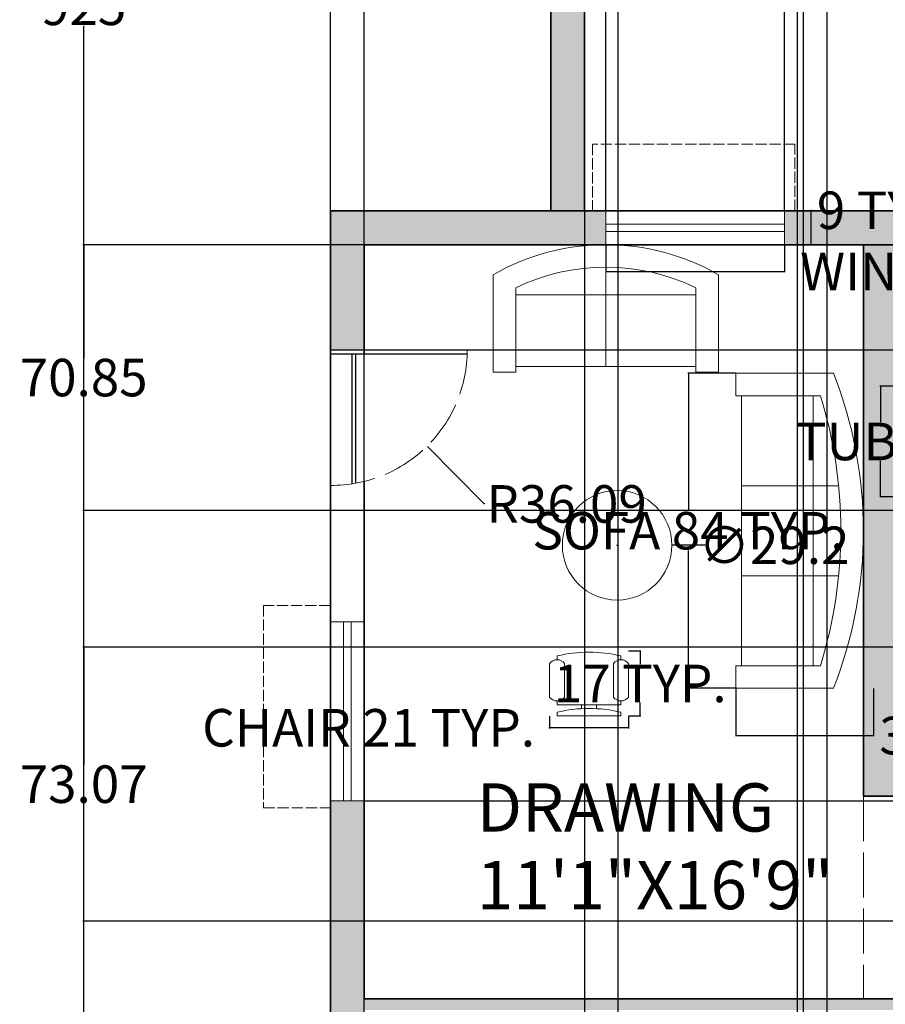
# Model space of a CAD drawing. Units: inches. Extents: x 300 to 1007, y 2 to 1069.
# Tile 4 of 12: x 337 to 568, y 271 to 533. Entities that reach past the tile are written whole.
import ezdxf

# ---------------------------------------------------------------- set-up
doc = ezdxf.new("R2010")
doc.units = ezdxf.units.IN
doc.header["$MEASUREMENT"] = 0
doc.linetypes.add('ACAD_ISO02W100', pattern=[15, 12, -3])
for name, color, linetype, lineweight in [('A-ANNO-DIMS', 2, 'Continuous', 18), ('A-AREA-IDEN', 7, 'Continuous', 18), ('A-DOOR', 3, 'Continuous', 25), ('A-DOOR-SWNG', 3, 'ACAD_ISO02W100', 13), ('A-FLOR-SLAB', 7, 'Continuous', 35), ('A-FURN', 8, 'Continuous', 18), ('A-GLAZ', 4, 'Continuous', 18), ('A-GLAZ-OVHD', 8, 'ACAD_ISO02W100', 13), ('A-WALL', 7, 'Continuous', 35), ('A-WALL-OVHD', 8, 'ACAD_ISO02W100', 18)]:
    doc.layers.add(name, color=color, linetype=linetype, lineweight=lineweight)
doc.layers.add('A-WALL-PATT', color=9, linetype='Continuous', lineweight=9, true_color=0xc7c8ca)
doc.styles.get("Standard").update_dxf_attribs({"font": 'arial.ttf'})
doc.dimstyles.get("Standard").update_dxf_attribs({"dimtxt": 10, "dimasz": 0.18, "dimexe": 0.18, "dimexo": 0.0625, "dimgap": 0.09, "dimtad": 0, "dimtih": 1, "dimtoh": 1, "dimdec": 0, "dimzin": 0, "dimdsep": 46, "dimlunit": 3, "dimtxsty": 'Standard', "dimcen": 0.09, "dimadec": 0, "dimazin": 0, "dimtfac": 1, "dimtdec": 0, "dimtofl": 0, "dimtmove": 0, "dimatfit": 3, "dimfxl": 1, "dimtolj": 1, "dimtzin": 0, "dimarcsym": 0})

# ---------------------------------------------------------------- blocks, each defined once
blk = doc.blocks.new('Chair - Desk')
for p, q in [((-8.5, 0), (-8.5, -1)), ((-8.5, 0), (8.5, 0)), ((8.5, 0), (8.5, -1)), ((-2, -3), (-2, -1.9355)), ((2, -1.9576), (2, -3)), ((-10.5, -5), (-10.5, -14)), ((-8.5, -3), (-8.5, -4)), ((-8.5, -3), (8.5, -3)), ((-6.5, -14), (-6.5, -5)), ((6.5, -5), (6.5, -14)), ((8.5, -3), (8.5, -4)), ((10.5, -14), (10.5, -5)), ((-8.5, -15), (-8.5, -16)), ((8.5, -15), (8.5, -16))]:
    blk.add_line(p, q)
for centre, radius, start, end in [((0, 34.625), 36.625, 256.5803, 283.4197), ((-8.5, -6.5), 2.5, 36.8699, 143.1301), ((8.5, -6.5), 2.5, 36.8699, 143.1301), ((-8.5, -12.5), 2.5, 216.8699, 323.1301), ((8.5, -12.5), 2.5, 216.8699, 323.1301), ((0, 19.625), 36.625, 256.5803, 283.4197)]:
    blk.add_arc(centre, radius, start, end)
blk = doc.blocks.new('Sofa - Roundback Loveseat 5 ft.')
for p, q in [((0, -32.44198), (0, -5.99998)), ((-24, -33.99998), (-24, -11.46958)), ((24.00004, -33.99998), (24.00004, -11.46958)), ((-23.9998, -13.38178), (23.99986, -13.38178)), ((-24, -32.44198), (24.00004, -32.44198))]:
    blk.add_line(p, q)
for points in [[(-24, -33.99998), (-30, -33.99998), (-30, -7.99998)], [(30.00004, -7.99998), (30.00004, -33.99998), (24.00004, -33.99998)]]:
    blk.add_lwpolyline(points)
for centre, radius, start, end in [((0, -60.24998), 60.24998, 60.13715, 119.8628), ((0, -61.38438), 55.38444, 64.32083, 115.6792)]:
    blk.add_arc(centre, radius, start, end)
blk = doc.blocks.new('Sofa - Roundback 7 ft.')
for p, q in [((-12.00002, -32.4421), (-12.00003, -6.5971)), ((11.99997, -32.4421), (11.99998, -6.5971)), ((-36.000027, -34), (-36.000027, -11.4696)), ((35.99998, -34), (35.99998, -11.4696)), ((-35.999844, -13.3819), (35.9998, -13.3819)), ((-36.000027, -32.4421), (35.99998, -32.4421))]:
    blk.add_line(p, q)
for points in [[(-36.000027, -34), (-42.000027, -34), (-42.000027, -8)], [(41.99998, -8), (41.99998, -34), (35.99998, -34)]]:
    blk.add_lwpolyline(points)
for centre, radius, start, end in [((0, -114.25), 114.25, 68.43141, 111.5686), ((-0.00001, -127.1968), 121.1968, 72.72033, 107.2797)]:
    blk.add_arc(centre, radius, start, end)
blk = doc.blocks.new('WIN-48')
for p, q in [((-47.83, 0), (-47.83, 4.5)), ((-47.83, 4.5), (-47.83, -4.5)), ((0, 4.5), (0, -4.5)), ((0, 1), (-47.83, 1)), ((0, -1), (-47.83, -1))]:
    blk.add_line(p, q)
blk = doc.blocks.new('WIN-47_5-8')
for p, q in [((-47.61, 0), (-47.61, 4.5)), ((-47.61, 4.5), (-47.61, -4.5)), ((0, -4.5), (0, 4.5)), ((0, 1), (-47.61, 1)), ((0, -1), (-47.61, -1))]:
    blk.add_line(p, q)
blk = doc.blocks.new('WINDOW-HOOD-54')
at = {"ltscale": 0.25}
for p, q in [((0, 17.83), (-53.97, 17.83)), ((-53.97, 17.83), (-53.97, 0)), ((0, 0), (0, 17.83))]:
    blk.add_line(p, q, dxfattribs=at)
blk = doc.blocks.new('*D21')
at = {"layer": 'A-ANNO-DIMS', "color": 0, "lineweight": -2, "transparency": 16777216}
for p, q in [((478.51, 347.69), (478.51, 344.42)), ((499.51, 347.69), (499.51, 344.42)), ((478.51, 344.6), (478.33, 344.6)), ((499.33, 344.6), (478.69, 344.6))]:
    blk.add_line(p, q, dxfattribs=at)
at = {"layer": 'A-ANNO-DIMS', "color": 0, "transparency": 16777216}
for points in [[(478.69, 344.63), (478.69, 344.57), (478.51, 344.6)], [(499.33, 344.63), (499.33, 344.57), (499.51, 344.6)]]:
    blk.add_solid(points, dxfattribs=at)
at = {"layer": 'Defpoints', "color": 0, "transparency": 16777216}
for p in [(478.51, 347.75), (499.51, 347.75), (478.51, 344.6)]:
    blk.add_point(p, dxfattribs=at)
at = {"layer": 'A-ANNO-DIMS', "color": 0, "transparency": 16777216, "insert": (430.29, 344.6), "char_height": 10, "attachment_point": 5}
blk.add_mtext('\\A1;CHAIR 21 TYP.', dxfattribs=at)
blk = doc.blocks.new('*D22')
at = {"layer": 'A-ANNO-DIMS', "color": 0, "lineweight": -2, "transparency": 16777216}
for p, q in [((499.57, 365.08), (502.84, 365.08)), ((502.66, 364.9), (502.66, 361.53)), ((502.66, 347.93), (502.66, 351.3)), ((499.57, 347.75), (502.84, 347.75))]:
    blk.add_line(p, q, dxfattribs=at)
at = {"layer": 'A-ANNO-DIMS', "color": 0, "transparency": 16777216}
for points in [[(502.63, 364.9), (502.69, 364.9), (502.66, 365.08)], [(502.63, 347.93), (502.69, 347.93), (502.66, 347.75)]]:
    blk.add_solid(points, dxfattribs=at)
at = {"layer": 'Defpoints', "color": 0, "transparency": 16777216}
for p in [(499.51, 365.08), (499.51, 347.75), (502.66, 347.75)]:
    blk.add_point(p, dxfattribs=at)
at = {"layer": 'A-ANNO-DIMS', "color": 0, "transparency": 16777216, "insert": (502.66, 356.42), "char_height": 10, "attachment_point": 5}
blk.add_mtext('\\A1;17 TYP.', dxfattribs=at)
blk = doc.blocks.new('*D35')
at = {"layer": 'A-ANNO-DIMS', "color": 0, "lineweight": -2, "transparency": 16777216}
for p, q in [((571.06, 435.66), (566.52, 435.66)), ((566.7, 435.48), (566.7, 426.11)), ((566.7, 406.35), (566.7, 415.72)), ((571.06, 406.17), (566.52, 406.17))]:
    blk.add_line(p, q, dxfattribs=at)
at = {"layer": 'A-ANNO-DIMS', "color": 0, "transparency": 16777216}
for points in [[(566.67, 435.48), (566.73, 435.48), (566.7, 435.66)], [(566.67, 406.35), (566.73, 406.35), (566.7, 406.17)]]:
    blk.add_solid(points, dxfattribs=at)
at = {"layer": 'Defpoints', "color": 0, "transparency": 16777216}
for p in [(571.12, 435.66), (566.7, 406.17), (571.12, 406.17)]:
    blk.add_point(p, dxfattribs=at)
at = {"layer": 'A-ANNO-DIMS', "color": 0, "transparency": 16777216, "insert": (566.7, 420.92), "char_height": 10, "attachment_point": 5}
blk.add_mtext('\\A1;TUB 29', dxfattribs=at)
blk = doc.blocks.new('*D51')
at = {"layer": 'A-ANNO-DIMS', "color": 0, "lineweight": -2, "transparency": 16777216}
for p, q in [((528.06, 439.13), (515.34, 439.13)), ((515.52, 438.95), (515.52, 402.39)), ((515.52, 355.31), (515.52, 391.86)), ((528.06, 355.13), (515.34, 355.13))]:
    blk.add_line(p, q, dxfattribs=at)
at = {"layer": 'A-ANNO-DIMS', "color": 0, "transparency": 16777216}
for points in [[(515.49, 438.95), (515.55, 438.95), (515.52, 439.13)], [(515.49, 355.31), (515.55, 355.31), (515.52, 355.13)]]:
    blk.add_solid(points, dxfattribs=at)
at = {"layer": 'Defpoints', "color": 0, "transparency": 16777216}
for p in [(528.12, 439.13), (515.52, 355.13), (528.12, 355.13)]:
    blk.add_point(p, dxfattribs=at)
at = {"layer": 'A-ANNO-DIMS', "color": 0, "transparency": 16777216, "insert": (515.52, 397.13), "char_height": 10, "attachment_point": 5}
blk.add_mtext('\\A1;SOFA 84 TYP.', dxfattribs=at)
blk = doc.blocks.new('*D52')
at = {"layer": 'A-ANNO-DIMS', "color": 0, "lineweight": -2, "transparency": 16777216}
for p, q in [((528.12, 355.06), (528.12, 342.35)), ((564.79, 355.06), (564.79, 342.35)), ((528.3, 342.53), (564.61, 342.53)), ((564.79, 342.53), (564.97, 342.53))]:
    blk.add_line(p, q, dxfattribs=at)
at = {"layer": 'A-ANNO-DIMS', "color": 0, "transparency": 16777216}
for points in [[(528.3, 342.56), (528.3, 342.5), (528.12, 342.53)], [(564.61, 342.56), (564.61, 342.5), (564.79, 342.53)]]:
    blk.add_solid(points, dxfattribs=at)
at = {"layer": 'Defpoints', "color": 0, "transparency": 16777216}
for p in [(528.12, 355.13), (564.79, 355.13), (564.79, 342.53)]:
    blk.add_point(p, dxfattribs=at)
at = {"layer": 'A-ANNO-DIMS', "color": 0, "transparency": 16777216, "insert": (589.39, 342.53), "char_height": 10, "attachment_point": 5}
blk.add_mtext('\\A1;37 TYP.', dxfattribs=at)
blk = doc.blocks.new('*D55')
at = {"layer": 'A-ANNO-DIMS', "color": 0, "lineweight": -2, "transparency": 16777216}
for p, q in [((493.48, 473.32), (493.48, 466.06)), ((541.08, 473.32), (541.08, 466.06)), ((493.66, 466.24), (540.9, 466.24)), ((541.08, 466.24), (541.26, 466.24))]:
    blk.add_line(p, q, dxfattribs=at)
at = {"layer": 'A-ANNO-DIMS', "color": 0, "transparency": 16777216}
for points in [[(493.66, 466.27), (493.66, 466.21), (493.48, 466.24)], [(540.9, 466.27), (540.9, 466.21), (541.08, 466.24)]]:
    blk.add_solid(points, dxfattribs=at)
at = {"layer": 'Defpoints', "color": 0, "transparency": 16777216}
for p in [(493.48, 473.38), (541.08, 473.38), (541.08, 466.24)]:
    blk.add_point(p, dxfattribs=at)
at = {"layer": 'A-ANNO-DIMS', "color": 0, "transparency": 16777216, "insert": (598.48, 466.24), "char_height": 10, "attachment_point": 5}
blk.add_mtext('\\A1;WINDOW 48 TYP.', dxfattribs=at)
blk = doc.blocks.new('*D56')
at = {"layer": 'A-ANNO-DIMS', "color": 0, "lineweight": -2, "transparency": 16777216}
for p, q in [((541.14, 482.38), (548.4, 482.38)), ((548.22, 482.38), (548.22, 482.56)), ((548.22, 482.56), (548.4, 482.56)), ((548.22, 473.56), (548.22, 482.2)), ((541.14, 473.38), (548.4, 473.38))]:
    blk.add_line(p, q, dxfattribs=at)
at = {"layer": 'A-ANNO-DIMS', "color": 0, "transparency": 16777216}
for points in [[(548.19, 482.2), (548.25, 482.2), (548.22, 482.38)], [(548.19, 473.56), (548.25, 473.56), (548.22, 473.38)]]:
    blk.add_solid(points, dxfattribs=at)
at = {"layer": 'Defpoints', "color": 0, "transparency": 16777216}
for p in [(541.08, 482.38), (548.22, 482.38), (541.08, 473.38)]:
    blk.add_point(p, dxfattribs=at)
at = {"layer": 'A-ANNO-DIMS', "color": 0, "transparency": 16777216, "insert": (568.95, 482.56), "char_height": 10, "attachment_point": 5}
blk.add_mtext('\\A1;9 TYP.', dxfattribs=at)
blk = doc.blocks.new('*D74')
at = {"layer": 'A-ANNO-DIMS', "color": 0, "lineweight": -2, "transparency": 16777216}
for p, q in [((478.76, 999.45), (354.19, 999.45)), ((354.37, 999.27), (354.37, 542.11)), ((354.37, 74.56), (354.37, 531.72)), ((420.06, 74.38), (354.19, 74.38))]:
    blk.add_line(p, q, dxfattribs=at)
at = {"layer": 'A-ANNO-DIMS', "color": 0, "transparency": 16777216}
for points in [[(354.34, 999.27), (354.4, 999.27), (354.37, 999.45)], [(354.34, 74.56), (354.4, 74.56), (354.37, 74.38)]]:
    blk.add_solid(points, dxfattribs=at)
at = {"layer": 'Defpoints', "color": 0, "transparency": 16777216}
for p in [(354.37, 999.45), (478.83, 999.45), (420.12, 74.38)]:
    blk.add_point(p, dxfattribs=at)
at = {"layer": 'A-ANNO-DIMS', "color": 0, "transparency": 16777216, "insert": (354.37, 536.92), "char_height": 10, "attachment_point": 5}
blk.add_mtext('\\A1;925', dxfattribs=at)
blk = doc.blocks.new('*D79')
at = {"layer": 'A-ANNO-DIMS', "color": 0, "lineweight": -2, "transparency": 16777216}
for p, q in [((420.12, 482.45), (420.12, 1063.03)), ((420.3, 1062.85), (436.4, 1062.85)), ((478.65, 1062.85), (462.55, 1062.85)), ((478.83, 482.45), (478.83, 1063.03))]:
    blk.add_line(p, q, dxfattribs=at)
at = {"layer": 'A-ANNO-DIMS', "color": 0, "transparency": 16777216}
for points in [[(420.3, 1062.88), (420.3, 1062.82), (420.12, 1062.85)], [(478.65, 1062.88), (478.65, 1062.82), (478.83, 1062.85)]]:
    blk.add_solid(points, dxfattribs=at)
at = {"layer": 'Defpoints', "color": 0, "transparency": 16777216}
for p in [(478.83, 1062.85), (420.12, 482.38), (478.83, 482.38)]:
    blk.add_point(p, dxfattribs=at)
at = {"layer": 'A-ANNO-DIMS', "color": 0, "transparency": 16777216, "insert": (449.47, 1062.85), "char_height": 10, "attachment_point": 5}
blk.add_mtext('\\A1;58.7', dxfattribs=at)
blk = doc.blocks.new('*D88')
at = {"layer": 'A-ANNO-DIMS', "color": 0, "lineweight": -2, "transparency": 16777216}
for p, q in [((429.12, 83.45), (429.12, 1063.03)), ((429.3, 1062.85), (445.92, 1062.85)), ((496.59, 1062.85), (479.97, 1062.85)), ((496.77, 83.45), (496.77, 1063.03))]:
    blk.add_line(p, q, dxfattribs=at)
at = {"layer": 'A-ANNO-DIMS', "color": 0, "transparency": 16777216}
for points in [[(429.3, 1062.88), (429.3, 1062.82), (429.12, 1062.85)], [(496.59, 1062.88), (496.59, 1062.82), (496.77, 1062.85)]]:
    blk.add_solid(points, dxfattribs=at)
at = {"layer": 'Defpoints', "color": 0, "transparency": 16777216}
for p in [(496.77, 1062.85), (429.12, 83.38), (496.77, 83.38)]:
    blk.add_point(p, dxfattribs=at)
at = {"layer": 'A-ANNO-DIMS', "color": 0, "transparency": 16777216, "insert": (462.95, 1062.85), "char_height": 10, "attachment_point": 5}
blk.add_mtext('\\A1;67.65', dxfattribs=at)
blk = doc.blocks.new('*D89')
at = {"layer": 'A-ANNO-DIMS', "color": 0, "lineweight": -2, "transparency": 16777216}
for p, q in [((544.6, 83.45), (544.6, 1063.03)), ((544.78, 1062.85), (554.56, 1062.85)), ((598.25, 1062.85), (588.48, 1062.85)), ((598.43, 83.45), (598.43, 1063.03))]:
    blk.add_line(p, q, dxfattribs=at)
at = {"layer": 'A-ANNO-DIMS', "color": 0, "transparency": 16777216}
for points in [[(544.78, 1062.88), (544.78, 1062.82), (544.6, 1062.85)], [(598.25, 1062.88), (598.25, 1062.82), (598.43, 1062.85)]]:
    blk.add_solid(points, dxfattribs=at)
at = {"layer": 'Defpoints', "color": 0, "transparency": 16777216}
for p in [(598.43, 1062.85), (544.6, 83.38), (598.43, 83.38)]:
    blk.add_point(p, dxfattribs=at)
at = {"layer": 'A-ANNO-DIMS', "color": 0, "transparency": 16777216, "insert": (571.52, 1062.85), "char_height": 10, "attachment_point": 5}
blk.add_mtext('\\A1;53.83', dxfattribs=at)
blk = doc.blocks.new('*D91')
at = {"layer": 'A-ANNO-DIMS', "color": 0, "lineweight": -2, "transparency": 16777216}
for p, q in [((429.18, 325.09), (974.48, 325.09)), ((974.3, 324.91), (974.3, 290.23)), ((974.3, 245.16), (974.3, 279.84)), ((429.18, 244.98), (974.48, 244.98))]:
    blk.add_line(p, q, dxfattribs=at)
at = {"layer": 'A-ANNO-DIMS', "color": 0, "transparency": 16777216}
for points in [[(974.27, 324.91), (974.33, 324.91), (974.3, 325.09)], [(974.27, 245.16), (974.33, 245.16), (974.3, 244.98)]]:
    blk.add_solid(points, dxfattribs=at)
at = {"layer": 'Defpoints', "color": 0, "transparency": 16777216}
for p in [(429.12, 325.09), (974.3, 325.09), (429.12, 244.98)]:
    blk.add_point(p, dxfattribs=at)
at = {"layer": 'A-ANNO-DIMS', "color": 0, "transparency": 16777216, "insert": (974.3, 285.04), "char_height": 10, "attachment_point": 5}
blk.add_mtext('\\A1;80.11', dxfattribs=at)
blk = doc.blocks.new('*D92')
at = {"layer": 'A-ANNO-DIMS', "color": 0, "lineweight": -2, "transparency": 16777216}
for p, q in [((429.18, 473.38), (974.48, 473.38)), ((974.3, 473.2), (974.3, 464.54)), ((974.3, 445.49), (974.3, 454.15)), ((429.18, 445.31), (974.48, 445.31))]:
    blk.add_line(p, q, dxfattribs=at)
at = {"layer": 'A-ANNO-DIMS', "color": 0, "transparency": 16777216}
for points in [[(974.27, 473.2), (974.33, 473.2), (974.3, 473.38)], [(974.27, 445.49), (974.33, 445.49), (974.3, 445.31)]]:
    blk.add_solid(points, dxfattribs=at)
at = {"layer": 'Defpoints', "color": 0, "transparency": 16777216}
for p in [(429.12, 473.38), (429.12, 445.31), (974.3, 445.31)]:
    blk.add_point(p, dxfattribs=at)
at = {"layer": 'A-ANNO-DIMS', "color": 0, "transparency": 16777216, "insert": (974.3, 459.35), "char_height": 10, "attachment_point": 5}
blk.add_mtext('\\A1;28.07', dxfattribs=at)
blk = doc.blocks.new('*D95')
at = {"layer": 'A-ANNO-DIMS', "color": 0, "lineweight": -2, "transparency": 16777216}
for p, q in [((901.06, 473.38), (354.19, 473.38)), ((354.37, 473.2), (354.37, 443.16)), ((354.37, 402.72), (354.37, 432.77)), ((901.06, 402.54), (354.19, 402.54))]:
    blk.add_line(p, q, dxfattribs=at)
at = {"layer": 'A-ANNO-DIMS', "color": 0, "transparency": 16777216}
for points in [[(354.34, 473.2), (354.4, 473.2), (354.37, 473.38)], [(354.34, 402.72), (354.4, 402.72), (354.37, 402.54)]]:
    blk.add_solid(points, dxfattribs=at)
at = {"layer": 'Defpoints', "color": 0, "transparency": 16777216}
for p in [(354.37, 473.38), (901.12, 473.38), (901.12, 402.54)]:
    blk.add_point(p, dxfattribs=at)
at = {"layer": 'A-ANNO-DIMS', "color": 0, "transparency": 16777216, "insert": (354.37, 437.96), "char_height": 10, "attachment_point": 5}
blk.add_mtext('\\A1;70.85', dxfattribs=at)
blk = doc.blocks.new('*D96')
at = {"layer": 'A-ANNO-DIMS', "color": 0, "lineweight": -2, "transparency": 16777216}
for p, q in [((901.06, 366.1), (354.19, 366.1)), ((354.37, 365.92), (354.37, 334.77)), ((354.37, 293.21), (354.37, 324.37)), ((901.06, 293.03), (354.19, 293.03))]:
    blk.add_line(p, q, dxfattribs=at)
at = {"layer": 'A-ANNO-DIMS', "color": 0, "transparency": 16777216}
for points in [[(354.34, 365.92), (354.4, 365.92), (354.37, 366.1)], [(354.34, 293.21), (354.4, 293.21), (354.37, 293.03)]]:
    blk.add_solid(points, dxfattribs=at)
at = {"layer": 'Defpoints', "color": 0, "transparency": 16777216}
for p in [(354.37, 366.1), (901.12, 366.1), (901.12, 293.03)]:
    blk.add_point(p, dxfattribs=at)
at = {"layer": 'A-ANNO-DIMS', "color": 0, "transparency": 16777216, "insert": (354.37, 329.57), "char_height": 10, "attachment_point": 5}
blk.add_mtext('\\A1;73.07', dxfattribs=at)
blk = doc.blocks.new('*D97')
at = {"layer": 'A-ANNO-DIMS', "color": 0, "lineweight": -2, "transparency": 16777216}
for p, q in [((487.83, 482.45), (487.83, 1063.03)), ((488.01, 1062.85), (493.3, 1062.85)), ((493.48, 482.45), (493.48, 1063.03)), ((493.48, 1062.85), (493.66, 1062.85))]:
    blk.add_line(p, q, dxfattribs=at)
at = {"layer": 'A-ANNO-DIMS', "color": 0, "transparency": 16777216}
for points in [[(488.01, 1062.88), (488.01, 1062.82), (487.83, 1062.85)], [(493.3, 1062.88), (493.3, 1062.82), (493.48, 1062.85)]]:
    blk.add_solid(points, dxfattribs=at)
at = {"layer": 'Defpoints', "color": 0, "transparency": 16777216}
for p in [(493.48, 1062.85), (487.83, 482.38), (493.48, 482.38)]:
    blk.add_point(p, dxfattribs=at)
at = {"layer": 'A-ANNO-DIMS', "color": 0, "transparency": 16777216, "insert": (510.63, 1062.85), "char_height": 10, "attachment_point": 5}
blk.add_mtext('\\A1;5.649', dxfattribs=at)
blk = doc.blocks.new('*D98')
at = {"layer": 'A-ANNO-DIMS', "color": 0, "lineweight": -2, "transparency": 16777216}
for p, q in [((541.08, 482.45), (541.08, 1063.03)), ((541.26, 1062.85), (543.81, 1062.85)), ((580.35, 1062.85), (577.8, 1062.85)), ((580.53, 482.45), (580.53, 1063.03))]:
    blk.add_line(p, q, dxfattribs=at)
at = {"layer": 'A-ANNO-DIMS', "color": 0, "transparency": 16777216}
for points in [[(541.26, 1062.88), (541.26, 1062.82), (541.08, 1062.85)], [(580.35, 1062.88), (580.35, 1062.82), (580.53, 1062.85)]]:
    blk.add_solid(points, dxfattribs=at)
at = {"layer": 'Defpoints', "color": 0, "transparency": 16777216}
for p in [(580.53, 1062.85), (541.08, 482.38), (580.53, 482.38)]:
    blk.add_point(p, dxfattribs=at)
at = {"layer": 'A-ANNO-DIMS', "color": 0, "transparency": 16777216, "insert": (560.81, 1062.85), "char_height": 10, "attachment_point": 5}
blk.add_mtext('\\A1;39.45', dxfattribs=at)
blk = doc.blocks.new('*D101')
at = {"layer": 'A-ANNO-DIMS', "color": 0, "lineweight": -2, "transparency": 16777216}
for p, q in [((487.83, 609.38), (487.83, 8.45)), ((552.34, 609.38), (552.34, 8.45)), ((488.01, 8.63), (504.06, 8.63)), ((552.16, 8.63), (536.11, 8.63))]:
    blk.add_line(p, q, dxfattribs=at)
at = {"layer": 'A-ANNO-DIMS', "color": 0, "transparency": 16777216}
for points in [[(488.01, 8.66), (488.01, 8.6), (487.83, 8.63)], [(552.16, 8.66), (552.16, 8.6), (552.34, 8.63)]]:
    blk.add_solid(points, dxfattribs=at)
at = {"layer": 'Defpoints', "color": 0, "transparency": 16777216}
for p in [(487.83, 609.45), (552.34, 609.45), (552.34, 8.63)]:
    blk.add_point(p, dxfattribs=at)
at = {"layer": 'A-ANNO-DIMS', "color": 0, "transparency": 16777216, "insert": (520.08, 8.63), "char_height": 10, "attachment_point": 5}
blk.add_mtext('\\A1;64.51', dxfattribs=at)
blk = doc.blocks.new('*D105')
at = {"layer": 'A-ANNO-DIMS', "color": 0, "lineweight": -2, "transparency": 16777216}
for p, q in [((487.83, 990.38), (487.83, 8.45)), ((546.1, 990.38), (546.1, 8.45)), ((488.01, 8.63), (499.99, 8.63)), ((545.92, 8.63), (533.94, 8.63))]:
    blk.add_line(p, q, dxfattribs=at)
at = {"layer": 'A-ANNO-DIMS', "color": 0, "transparency": 16777216}
for points in [[(488.01, 8.66), (488.01, 8.6), (487.83, 8.63)], [(545.92, 8.66), (545.92, 8.6), (546.1, 8.63)]]:
    blk.add_solid(points, dxfattribs=at)
at = {"layer": 'Defpoints', "color": 0, "transparency": 16777216}
for p in [(487.83, 990.45), (546.1, 990.45), (546.1, 8.63)]:
    blk.add_point(p, dxfattribs=at)
at = {"layer": 'A-ANNO-DIMS', "color": 0, "transparency": 16777216, "insert": (516.97, 8.63), "char_height": 10, "attachment_point": 5}
blk.add_mtext('\\A1;58.28', dxfattribs=at)
blk = doc.blocks.new('*D109')
at = {"layer": 'A-ANNO-DIMS', "color": 0, "lineweight": -2, "transparency": 16777216}
for p, q in [((496.42, 393.25), (496.6, 393.25)), ((496.51, 393.16), (496.51, 393.34)), ((519.87, 393.25), (511.29, 393.25))]:
    blk.add_line(p, q, dxfattribs=at)
at = {"layer": 'A-ANNO-DIMS', "color": 0, "transparency": 16777216}
blk.add_solid([(511.29, 393.28), (511.29, 393.22), (511.11, 393.25)], dxfattribs=at)
at = {"layer": 'Defpoints', "color": 0, "transparency": 16777216}
for p in [(481.91, 393.25), (511.11, 393.25)]:
    blk.add_point(p, dxfattribs=at)
at = {"layer": 'A-ANNO-DIMS', "color": 0, "transparency": 16777216, "insert": (538.33, 393.25), "char_height": 10, "attachment_point": 5}
blk.add_mtext('\\A1;∅29.2', dxfattribs=at)
blk = doc.blocks.new('*D111')
at = {"layer": 'A-ANNO-DIMS', "color": 0, "lineweight": -2, "transparency": 16777216}
for p, q in [((420.38, 445.31), (420.56, 445.31)), ((420.47, 445.22), (420.47, 445.4)), ((461.11, 404.28), (445.99, 419.54)), ((461.29, 404.28), (461.11, 404.28))]:
    blk.add_line(p, q, dxfattribs=at)
at = {"layer": 'A-ANNO-DIMS', "color": 0, "transparency": 16777216}
blk.add_solid([(446.01, 419.56), (445.97, 419.52), (445.87, 419.67)], dxfattribs=at)
at = {"layer": 'Defpoints', "color": 0, "transparency": 16777216}
for p in [(420.47, 445.31), (445.87, 419.67)]:
    blk.add_point(p, dxfattribs=at)
at = {"layer": 'A-ANNO-DIMS', "color": 0, "transparency": 16777216, "insert": (483.04, 404.28), "char_height": 10, "attachment_point": 5}
blk.add_mtext('\\A1;R36.09', dxfattribs=at)

msp = doc.modelspace()

# ---------------------------------------------------------------- hatches: boundary and pattern name
at = {"layer": 'A-WALL-PATT'}
h = msp.add_hatch(color=256, dxfattribs=at)
h.dxf.hatch_style = 1
h.paths.add_polyline_path([(546.104, 999.4468), (478.8267, 999.4468), (478.8267, 869.2798, -0.06322715), (487.8267, 868.1328), (487.8267, 990.4468), (546.104, 990.4468)])
h.paths.add_polyline_path([(630.4852, 999.4468), (582.106, 999.4468), (582.106, 990.4468), (613.8267, 990.4468), (613.8267, 867.4468), (622.8267, 867.4468), (622.8267, 990.4468), (630.4852, 990.4468)])
h.paths.add_polyline_path([(702.0883, 999.4468), (650.4653, 999.4468), (650.4653, 990.4468), (682.8267, 990.4468), (682.8267, 960.0824, -0.02530575), (685.8267, 960.0478), (685.8267, 990.4468), (702.0883, 990.4468)])
h.paths.add_polyline_path([(850.8267, 999.4468), (737.5888, 999.4468), (737.5888, 990.4468), (841.8267, 990.4468), (841.8267, 950.5685), (850.8267, 950.5685)])
h.paths.add_polyline_path([(685.8267, 930.4465), (682.8267, 930.4465), (682.8267, 888.4468), (682.8267, 867.4468), (685.8267, 867.4468), (697.4169, 867.4468), (697.4169, 870.4468), (685.8267, 870.4468), (685.8267, 888.4468)])
h.paths.add_polyline_path([(682.8267, 931.4465), (654.3436, 931.4465, 0.00843109), (654.3267, 930.4465), (682.8267, 930.4465)])
h.paths.add_polyline_path([(685.8267, 931.4465), (682.8267, 931.4465), (682.8267, 930.4465), (685.8267, 930.4465)])
h.paths.add_polyline_path([(682.8267, 888.4468), (622.8267, 888.4468), (622.8267, 885.4468), (682.8267, 885.4468)])
h.paths.add_polyline_path([(850.8267, 870.4468), (850.8267, 914.7851), (841.8267, 914.7851), (841.8267, 870.4468), (732.7101, 870.4468, -0.02120595), (732.8267, 867.4468), (779.8267, 867.4468), (779.8267, 749.4468), (782.8267, 749.4468), (788.8267, 749.4468), (788.8267, 861.4468), (841.8267, 861.4468), (841.8267, 749.4468), (850.8267, 749.4468)])
h.paths.add_polyline_path([(622.8267, 810.4468), (487.8267, 810.4468), (487.8267, 833.2626), (478.8267, 833.2626), (478.8267, 609.4468), (478.8267, 482.3847), (487.8267, 482.3847), (487.8267, 801.4468), (620.8267, 801.4468), (622.8267, 801.4468)])
h.paths.add_polyline_path([(680.8267, 729.4468), (620.8267, 729.4468), (620.8267, 765.8246, -0.02111352), (617.8267, 766.0562), (617.8267, 698.7303), (620.8267, 698.7303), (620.8267, 726.4468), (680.8267, 726.4468)])
h.paths.add_polyline_path([(620.8267, 668.8122, -0.02498293), (617.8267, 668.6448), (617.8267, 618.4468), (600.3357, 618.4468), (600.3357, 609.4468), (652.9929, 609.4468), (652.9929, 618.4468), (620.8267, 618.4468)])
h.paths.add_polyline_path([(552.3393, 618.4468), (487.8267, 618.4468), (487.8267, 609.4468), (552.3393, 609.4468)], flags=17)
h.paths.add_polyline_path([(694.5763, 618.4468), (683.8267, 618.4468), (683.8267, 726.4468), (683.8267, 749.4468), (680.8267, 749.4468), (680.8267, 740.4468), (680.8267, 726.4468), (680.8267, 618.4468), (674.1573, 618.4468), (674.1573, 609.4468), (680.8267, 609.4468), (694.5763, 609.4468)])
h.paths.add_polyline_path([(850.8267, 642.8902), (841.8267, 642.8902), (841.8267, 618.4468), (782.8267, 618.4468), (782.8267, 708.0513, -0.02308839), (779.8267, 707.9092), (779.8267, 618.4468), (730.1068, 618.4468), (730.1068, 609.4468), (779.8267, 609.4468), (841.8267, 609.4468), (841.8267, 482.3847), (850.8267, 482.3847)])
h.paths.add_polyline_path([(850.8267, 749.4468), (841.8267, 749.4468), (841.8267, 705.9119), (850.8267, 705.9119)])
h.paths.add_polyline_path([(841.8267, 749.4468), (782.8267, 749.4468), (779.8267, 749.4468), (761.9959, 749.4468), (761.9959, 740.4468), (779.8267, 740.4468), (812.3267, 740.4468), (841.8267, 740.4468)])
h.paths.add_polyline_path([(669.1457, 482.3847), (604.489, 482.3847), (604.489, 473.3847), (631.1217, 473.3847), (631.1217, 436.0244, -0.02504709), (634.1217, 436.1748), (634.1217, 436.4367), (634.1217, 473.3847), (669.1457, 473.3847)], flags=17)
h.paths.add_polyline_path([(580.5305, 482.3847), (571.1217, 482.3847), (541.0813, 482.3847), (541.0813, 473.3847), (562.1217, 473.3847), (562.1217, 326.3847), (571.1217, 326.3847), (571.1217, 362.3847), (631.1217, 362.3847), (631.1217, 326.3847), (706.9024, 326.3847, -0.02105388), (706.9999, 329.3847), (634.1217, 329.3847), (634.1217, 365.3847), (634.1217, 406.1748), (631.1217, 406.1748), (631.1217, 365.3847), (571.1217, 365.3847), (571.1217, 473.3847), (580.5305, 473.3847)])
h.paths.add_polyline_path([(493.4756, 482.3847), (420.1217, 482.3847), (420.1217, 445.3134), (429.1217, 445.3134), (429.1217, 473.3847), (493.4756, 473.3847)])
h.paths.add_polyline_path([(786.2236, 482.3847), (716.7793, 482.3847), (716.7793, 473.3847), (766.1217, 473.3847), (766.1217, 329.3847), (742.5583, 329.3847), (742.5583, 326.3847), (766.1217, 326.3847), (766.1217, 316.0647), (769.1217, 316.0647), (769.1217, 326.3847), (769.1217, 473.3847), (786.2236, 473.3847)])
h.paths.add_polyline_path([(910.1217, 482.3847), (822.7166, 482.3847), (822.7166, 473.3847), (901.1217, 473.3847), (901.1217, 402.5393), (910.1217, 402.5393)])
h.paths.add_polyline_path([(910.1217, 366.1034), (901.1217, 366.1034), (901.1217, 329.3847), (814.1217, 329.3847), (814.1217, 312.5176), (817.1217, 312.5176), (817.1217, 326.3847), (901.1217, 326.3847), (901.1217, 293.0319), (910.1217, 293.0319), (910.1217, 326.3847)])
h.paths.add_polyline_path([(910.1217, 268.9355), (901.1217, 268.9355), (901.1217, 254.3847), (817.1217, 254.3847), (817.1217, 290.5411, -0.03396715), (814.1217, 290.3847), (814.1217, 254.3847), (775.1217, 254.3847), (775.1217, 281.5164), (769.1217, 281.5164), (769.1217, 292.1577), (766.1217, 292.1577), (766.1217, 254.3847), (766.1217, 220.1938), (775.5079, 220.1938), (775.5079, 251.3847), (817.1217, 251.3847), (901.1217, 251.3847), (901.1217, 152.3847), (819.0246, 152.3847, -0.02493798), (818.9117, 149.3847), (901.1217, 149.3847), (901.1217, 92.3847), (901.1217, 83.3847), (874.3528, 83.3847), (874.3528, 74.3847), (910.1217, 74.3847), (910.1217, 92.3847), (910.1217, 149.3847)])
h.paths.add_polyline_path([(429.1217, 325.0924), (420.1217, 325.0924), (420.1217, 263.3847), (420.1217, 244.9834), (429.1217, 244.9834), (429.1217, 269.3847), (571.1217, 269.3847), (571.1217, 272.3847), (562.1217, 272.3847), (429.1217, 272.3847)])
h.paths.add_polyline_path([(429.1217, 208.998), (420.1217, 208.998), (420.1217, 74.3847), (496.7704, 74.3847), (496.7704, 83.3847), (429.1217, 83.3847)])
h.paths.add_polyline_path([(598.4322, 83.3847), (571.1217, 83.3847), (571.1217, 122.1171), (562.1217, 122.1171), (562.1217, 83.3847), (544.6031, 83.3847), (544.6031, 74.3847), (598.4322, 74.3847)])
h.paths.add_polyline_path([(797.0822, 83.3847), (769.1217, 83.3847), (769.1217, 149.3847), (788.9123, 149.3847), (788.9123, 152.3847), (769.1217, 152.3847), (769.1217, 178.0167), (766.1217, 178.0167), (766.1217, 152.3847), (735.3598, 152.3847), (735.3598, 143.3847), (766.1217, 143.3847), (766.1217, 83.3847), (634.1217, 83.3847), (634.1217, 143.3847), (659.7326, 143.3847), (659.7326, 152.3847), (634.1217, 152.3847), (634.1217, 194.3847), (571.1217, 194.3847), (571.1217, 233.7289, -0.06379947), (562.1217, 234.7942), (562.1217, 163.4485), (567.7403, 163.4485), (567.7403, 152.3847), (571.1217, 152.3847), (571.1217, 191.3847), (631.1217, 191.3847), (631.1217, 83.3847), (621.979, 83.3847), (621.979, 74.3847), (631.1217, 74.3847), (797.0822, 74.3847)])

# ---------------------------------------------------------------- linework, layer by layer
at = {"layer": 'A-DOOR'}
for p, q in [((420.1217, 445.3134), (429.1217, 445.3134)), ((420.1217, 444.3134), (420.1217, 445.3134)), ((420.1217, 445.3134), (456.5612, 445.3134)), ((420.1217, 444.3134), (456.5612, 444.3134)), ((425.8349, 444.3134), (425.8349, 409.6228)), ((426.8349, 444.3134), (426.8349, 409.7875))]:
    msp.add_line(p, q, dxfattribs=at)
at = {"layer": 'A-DOOR-SWNG'}
msp.add_arc((420.4696, 445.3134), 36.0916, 269.44766, 0, dxfattribs=at)
at = {"layer": 'A-FLOR-SLAB'}
msp.add_line((478.8267, 482.3847), (478.8267, 609.4468), dxfattribs=at)
at = {"layer": 'A-FURN'}
msp.add_circle((496.5074, 393.2521), 14.6, dxfattribs=at)
at = {"layer": 'A-WALL'}
for p, q in [((487.8267, 801.4468), (487.8267, 482.3847)), ((631.1217, 326.3847), (562.1217, 326.3847)), ((562.1217, 272.3847), (571.1217, 272.3847))]:
    msp.add_line(p, q, dxfattribs=at)
for points in [[(571.1217, 482.3847), (420.1217, 482.3847), (420.1217, 263.3847)], [(562.1217, 326.3847), (562.1217, 473.3847), (429.1217, 473.3847), (429.1217, 444.3134)], [(429.1217, 410.2742), (429.1217, 272.3847), (562.1217, 272.3847)]]:
    msp.add_lwpolyline(points, dxfattribs=at)
at = {"layer": 'A-WALL-OVHD'}
msp.add_line((562.1217, 326.3847), (562.1217, 272.3847), dxfattribs=at)

# ---------------------------------------------------------------- block references
at = {"layer": 'A-FURN'}
msp.add_blockref('Sofa - Roundback Loveseat 5 ft.', (493.4756, 473.3847), dxfattribs=at)
for name, p, rotation in [('Sofa - Roundback 7 ft.', (562.1217, 397.126), 270), ('Chair - Desk', (489.0096, 347.7503), 180)]:
    msp.add_blockref(name, p, dxfattribs=dict(at, rotation=rotation))
at = {"layer": 'A-GLAZ'}
msp.add_blockref('WIN-47_5-8', (541.0813, 477.8847), dxfattribs=at)
at = {"layer": 'A-GLAZ', "extrusion": (0, 0, -1), "xscale": 0.999156112481668, "zscale": -1, "rotation": 90}
msp.add_blockref('WIN-48', (-424.6217, 372.8847), dxfattribs=at)
at = {"layer": 'A-GLAZ-OVHD'}
msp.add_blockref('WINDOW-HOOD-54', (543.8732, 482.3847), dxfattribs=at)
at = {"layer": 'A-GLAZ-OVHD', "rotation": 90.0000000000001}
msp.add_blockref('WINDOW-HOOD-54', (420.1217, 377.2398), dxfattribs=at)

# ---------------------------------------------------------------- texts
at = {"layer": 'A-AREA-IDEN'}
for s, height, p in [('DRAWING', 12.87594, (459.0983, 316.9198)), ('11\'1"X16\'9"', 12.875935, (459.0983, 296.2358))]:
    msp.add_text(s, height=height, dxfattribs=at).set_placement(p)

# ---------------------------------------------------------------- dimensions: what is measured, and where the dimension line sits
at = {"layer": 'A-ANNO-DIMS'}
for base, p1, p2, override, picture, middle in [((478.8267, 1062.8469), (420.1217, 482.3847), (478.8267, 482.3847), {"dimdec": 1, "dimlfac": 1, "dimrnd": 0, "dimzin": 0, "dimdsep": 46, "dimlunit": 2}, '*D79', (449.4742, 1062.8469)), ((496.7704, 1062.8469), (429.1217, 83.3847), (496.7704, 83.3847), {"dimdec": 2, "dimlfac": 1, "dimrnd": 0, "dimzin": 0, "dimdsep": 46, "dimlunit": 2}, '*D88', (462.946, 1062.8469)), ((493.4756, 1062.8469), (487.8267, 482.3847), (493.4756, 482.3847), {"dimdec": 3, "dimlfac": 1, "dimrnd": 0, "dimzin": 0, "dimdsep": 46, "dimlunit": 2}, '*D97', (510.6283, 1062.8469)), ((580.5305, 1062.8469), (541.0813, 482.3847), (580.5305, 482.3847), {"dimdec": 2, "dimlfac": 1, "dimrnd": 0, "dimzin": 0, "dimdsep": 46, "dimlunit": 2}, '*D98', (560.8059, 1062.8469)), ((598.4322, 1062.8469), (544.6031, 83.3847), (598.4322, 83.3847), {"dimdec": 2, "dimlfac": 1, "dimrnd": 0, "dimzin": 0, "dimdsep": 46, "dimlunit": 2}, '*D89', (571.5176, 1062.8469)), ((546.104, 8.6288), (487.8267, 990.4468), (546.104, 990.4468), {"dimdec": 2, "dimlfac": 1, "dimrnd": 0, "dimzin": 0, "dimdsep": 46, "dimlunit": 2}, '*D105', (516.9653, 8.6288)), ((552.3393, 8.6288), (487.8267, 609.4468), (552.3393, 609.4468), {"dimdec": 2, "dimlfac": 1, "dimrnd": 0, "dimzin": 0, "dimdsep": 46, "dimlunit": 2}, '*D101', (520.083, 8.6288))]:
    dim = msp.add_linear_dim(base=base, p1=p1, p2=p2, dimstyle='Standard', override=override, dxfattribs=at)
    dim.commit()
    dim.dimension.update_dxf_attribs({"geometry": picture, "text_midpoint": middle})
for base, p1, p2, override, picture, middle in [((354.3658, 999.4468), (420.1217, 74.3847), (478.8267, 999.4468), {"dimdec": 0, "dimlfac": 1, "dimrnd": 0, "dimzin": 0, "dimdsep": 46, "dimlunit": 2}, '*D74', (354.3658, 536.9158)), ((354.3658, 473.3847), (901.1217, 402.5393), (901.1217, 473.3847), {"dimdec": 2, "dimlfac": 1, "dimrnd": 0, "dimzin": 0, "dimdsep": 46, "dimlunit": 2}, '*D95', (354.3658, 437.962)), ((974.3023, 445.3134), (429.1217, 473.3847), (429.1217, 445.3134), {"dimdec": 2, "dimlfac": 1, "dimrnd": 0, "dimzin": 0, "dimdsep": 46, "dimlunit": 2}, '*D92', (974.3023, 459.3491)), ((354.3658, 366.1034), (901.1217, 293.0319), (901.1217, 366.1034), {"dimdec": 2, "dimlfac": 1, "dimrnd": 0, "dimzin": 0, "dimdsep": 46, "dimlunit": 2}, '*D96', (354.3658, 329.5676)), ((974.3023, 325.0924), (429.1217, 244.9834), (429.1217, 325.0924), {"dimdec": 2, "dimlfac": 1, "dimrnd": 0, "dimzin": 0, "dimdsep": 46, "dimlunit": 2}, '*D91', (974.3023, 285.0379))]:
    dim = msp.add_linear_dim(base=base, p1=p1, p2=p2, angle=90, dimstyle='Standard', override=override, dxfattribs=at)
    dim.commit()
    dim.dimension.update_dxf_attribs({"geometry": picture, "text_midpoint": middle})
for base, p1, p2, angle, text, picture, middle in [((548.2221, 482.3847), (541.0813, 473.3847), (541.0813, 482.3847), 90, '<> TYP.', '*D56', (568.9457, 482.5647)), ((515.5217, 355.126), (528.1217, 439.126), (528.1217, 355.126), 270, 'SOFA <> TYP.', '*D51', (515.5217, 397.126)), ((566.6987, 406.1748), (571.1217, 435.6613), (571.1217, 406.1748), 270, 'TUB <>', '*D35', (566.6987, 420.9181)), ((502.6596, 347.7503), (499.5096, 365.0837), (499.5096, 347.7503), 270, '<> TYP.', '*D22', (502.6596, 356.417)), ((478.5096, 344.6003), (499.5096, 347.7503), (478.5096, 347.7503), 180, 'CHAIR <> TYP.', '*D21', (430.286, 344.6003))]:
    dim = msp.add_linear_dim(base=base, p1=p1, p2=p2, angle=angle, text=text, dimstyle='Standard', override={"dimdec": 0, "dimlfac": 1, "dimrnd": 0, "dimzin": 0, "dimdsep": 46, "dimlunit": 2}, dxfattribs=at)
    dim.commit()
    dim.dimension.update_dxf_attribs({"geometry": picture, "text_midpoint": middle})
for base, p1, p2, text, picture, middle in [((541.0813, 466.2439), (493.4756, 473.3847), (541.0813, 473.3847), 'WINDOW <> TYP.', '*D55', (598.4829, 466.2439)), ((564.7884, 342.526), (528.1217, 355.126), (564.7884, 355.126), '<> TYP.', '*D52', (589.3933, 342.526))]:
    dim = msp.add_linear_dim(base=base, p1=p1, p2=p2, text=text, dimstyle='Standard', override={"dimdec": 0, "dimlfac": 1, "dimrnd": 0, "dimzin": 0, "dimdsep": 46, "dimlunit": 2}, dxfattribs=at)
    dim.commit()
    dim.dimension.update_dxf_attribs({"geometry": picture, "text_midpoint": middle})
dim = msp.add_radius_dim(center=(420.4696, 445.3134), mpoint=(445.8669, 419.6701), dimstyle='Standard', override={"dimdec": 2, "dimlfac": 1, "dimrnd": 0, "dimzin": 0, "dimdsep": 46, "dimlunit": 2}, dxfattribs=at)
dim.commit()
dim.dimension.update_dxf_attribs({"geometry": '*D111', "text_midpoint": (483.0431, 404.2841), "dimtype": 164})
dim = msp.add_diameter_dim_2p(p1=(481.9074, 393.2523), p2=(511.1073, 393.252), dimstyle='Standard', override={"dimdec": 1, "dimlfac": 1, "dimrnd": 0, "dimzin": 0, "dimdsep": 46, "dimlunit": 2}, dxfattribs=at)
dim.commit()
dim.dimension.update_dxf_attribs({"geometry": '*D109', "text_midpoint": (519.8673, 393.2519), "dimtype": 163})

doc.saveas('drawing.dxf')
